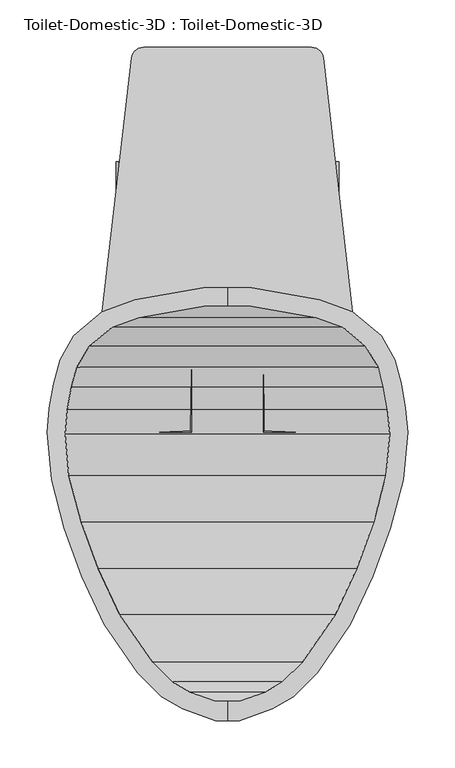
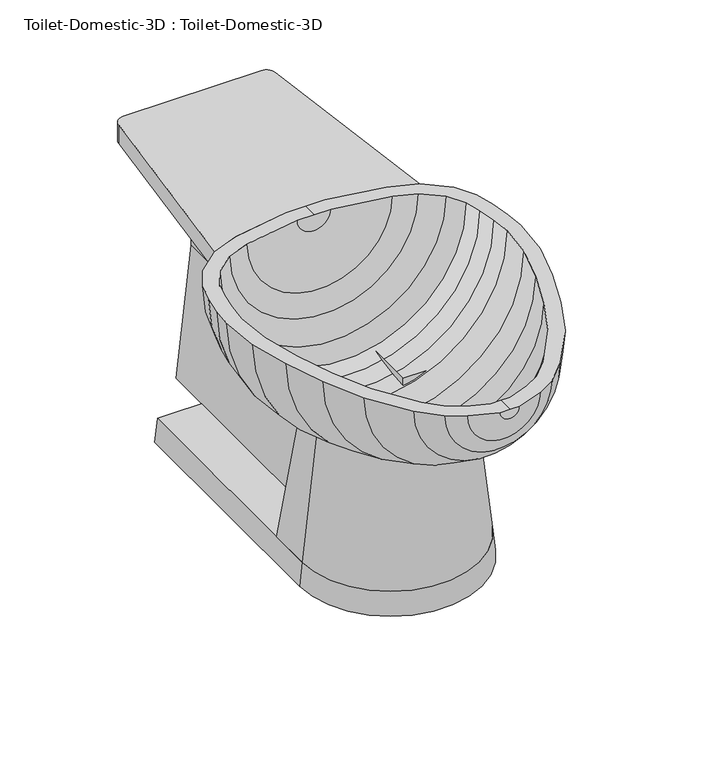
"""IFC4 building model written with IfcOpenShell, lengths in millimetres: flow terminal geometry, Toilet-Domestic-3D : Toilet-Domestic-3D."""

from ifc_helpers import new_model, si_unit, point, frame, frame_2d, origin, place, context, project, spatial, polyline, circle_curve, trimmed, segment, composite_curve, outline, extrude, source, transform, mapped, element, save
from ifc_brep_helpers import plane_surface, revolved_surface, advanced_brep


def toilet_domestic_3d_toilet_domestic_3d_ba6479b0(model_context):
    return source(origin(), model_context, "Body", "SolidModel", [
        advanced_brep(
        [(-25.4, 152.4, 361.95), (-97.4252791, 139.7, 361.95), (-132.3182423, 127.0, 361.95), (-162.5887836, 101.6, 361.95), (-176.9845865, 76.2, 361.95), (-183.790496, 50.8, 361.95), (-188.2862441, 25.3033453, 361.95), (-190.5, 0.0, 361.95), (-186.0724883, -50.6066907, 361.95), (-172.4088722, -101.6, 361.95), (-153.9191843, -152.4, 361.95), (-130.2307553, -203.2, 361.95), (-94.9900085, -254.0, 361.95), (-69.5900085, -279.4, 361.95), (-47.5929632, -292.1, 361.95), (-12.7, -304.8, 361.95), (0.0, -304.8, 361.95), (0.0, -284.592034, 361.95), (-12.5224565, -284.592034, 361.95), (-39.5113323, -274.7688865, 361.95), (-58.4178985, -263.8531754, 361.95), (-79.2146703, -243.0564036, 361.95), (-114.0255101, -192.8761202, 361.95), (-136.654021, -144.3491221, 361.95), (-154.575847, -95.1093097, 361.95), (-167.7238545, -46.0402777, 361.95), (-171.5645445, -2.1409906, 361.95), (-169.3087351, 23.6430284, 361.95), (-165.101298, 47.5045901, 361.95), (-159.5484355, 68.2281551, 361.95), (-146.1085923, 90.5605136, 361.95), (-121.9980886, 110.7916284, 361.95), (-94.1172813, 120.9394123, 361.95), (-22.0920022, 133.6394123, 361.95), (0.0, 133.6394123, 361.95), (0.0, 152.4, 361.95), (25.4, 152.4, 361.95), (22.0920022, 133.6394123, 361.95), (94.1172813, 120.9394123, 361.95), (121.9980886, 110.7916284, 361.95), (146.1085923, 90.5605136, 361.95), (159.5484355, 68.2281551, 361.95), (165.101298, 47.5045901, 361.95), (169.3087351, 23.6430284, 361.95), (171.5645445, -2.1409906, 361.95), (167.7238545, -46.0402777, 361.95), (154.575847, -95.1093097, 361.95), (136.654021, -144.3491221, 361.95), (114.0255101, -192.8761202, 361.95), (79.2146703, -243.0564036, 361.95), (58.4178985, -263.8531754, 361.95), (39.5113323, -274.7688865, 361.95), (12.5224565, -284.592034, 361.95), (12.7, -304.8, 361.95), (47.5929632, -292.1, 361.95), (69.5900085, -279.4, 361.95), (94.9900085, -254.0, 361.95), (130.2307553, -203.2, 361.95), (153.9191843, -152.4, 361.95), (172.4088722, -101.6, 361.95), (186.0724883, -50.6066907, 361.95), (190.5, 0.0, 361.95), (188.2862441, 25.3033453, 361.95), (183.790496, 50.8, 361.95), (176.9845865, 76.2, 361.95), (162.5887836, 101.6, 361.95), (132.3182423, 127.0, 361.95), (97.4252791, 139.7, 361.95)],
        [
            (0, 1),
            (1, 2),
            (2, 3),
            (3, 4),
            (4, 5),
            (5, 6),
            (6, 7),
            (7, 8),
            (8, 9),
            (9, 10),
            (10, 11),
            (11, 12),
            (12, 13),
            (13, 14),
            (14, 15),
            (15, 16),
            (16, 17),
            (17, 18),
            (18, 19),
            (19, 20),
            (20, 21),
            (21, 22),
            (22, 23),
            (23, 24),
            (24, 25),
            (25, 26),
            (26, 27),
            (27, 28),
            (28, 29),
            (29, 30),
            (30, 31),
            (31, 32),
            (32, 33),
            (33, 34),
            (34, 35),
            (35, 0),
            (36, 35),
            (34, 37),
            (37, 38),
            (38, 39),
            (39, 40),
            (40, 41),
            (41, 42),
            (42, 43),
            (43, 44),
            (44, 45),
            (45, 46),
            (46, 47),
            (47, 48),
            (48, 49),
            (49, 50),
            (50, 51),
            (51, 52),
            (52, 17),
            (16, 53),
            (53, 54),
            (54, 55),
            (55, 56),
            (56, 57),
            (57, 58),
            (58, 59),
            (59, 60),
            (60, 61),
            (61, 62),
            (62, 63),
            (63, 64),
            (64, 65),
            (65, 66),
            (66, 67),
            (67, 36),
            (67, 1, circle_curve(frame((0.0, 139.7, 361.95), z_axis=(0.0, 1.0, 0.0), x_axis=(-1.0, 0.0, 0.0)), 97.4252791)),
            (0, 36, circle_curve(frame((0.0, 152.4, 361.95), z_axis=(0.0, -1.0, 0.0), x_axis=(-1.0, 0.0, 0.0)), 25.4)),
            (66, 2, circle_curve(frame((0.0, 127.0, 361.95), z_axis=(0.0, 1.0, 0.0), x_axis=(-1.0, 0.0, 0.0)), 132.3182423)),
            (65, 3, circle_curve(frame((0.0, 101.6, 361.95), z_axis=(0.0, 1.0, 0.0), x_axis=(-1.0, 0.0, 0.0)), 162.5887836)),
            (64, 4, circle_curve(frame((0.0, 76.2, 361.95), z_axis=(0.0, 1.0, 0.0), x_axis=(-1.0, 0.0, 0.0)), 176.9845865)),
            (63, 5, circle_curve(frame((0.0, 50.8, 361.95), z_axis=(0.0, 1.0, 0.0), x_axis=(-1.0, 0.0, 0.0)), 183.790496)),
            (62, 6, circle_curve(frame((0.0, 25.3033453, 361.95), z_axis=(0.0, 1.0, 0.0), x_axis=(-1.0, 0.0, 0.0)), 188.2862441)),
            (61, 7, circle_curve(frame((0.0, 0.0, 361.95), z_axis=(0.0, 1.0, 0.0), x_axis=(-1.0, 0.0, 0.0)), 190.5)),
            (60, 8, circle_curve(frame((0.0, -50.6066907, 361.95), z_axis=(0.0, 1.0, 0.0), x_axis=(-1.0, 0.0, 0.0)), 186.0724883)),
            (59, 9, circle_curve(frame((0.0, -101.6, 361.95), z_axis=(0.0, 1.0, 0.0), x_axis=(-1.0, 0.0, 0.0)), 172.4088722)),
            (58, 10, circle_curve(frame((0.0, -152.4, 361.95), z_axis=(0.0, 1.0, 0.0), x_axis=(-1.0, 0.0, 0.0)), 153.9191843)),
            (57, 11, circle_curve(frame((0.0, -203.2, 361.95), z_axis=(0.0, 1.0, 0.0), x_axis=(-1.0, 0.0, 0.0)), 130.2307553)),
            (56, 12, circle_curve(frame((0.0, -254.0, 361.95), z_axis=(0.0, 1.0, 0.0), x_axis=(-1.0, 0.0, 0.0)), 94.9900085)),
            (55, 13, circle_curve(frame((0.0, -279.4, 361.95), z_axis=(0.0, 1.0, 0.0), x_axis=(-1.0, 0.0, 0.0)), 69.5900085)),
            (54, 14, circle_curve(frame((0.0, -292.1, 361.95), z_axis=(0.0, 1.0, 0.0), x_axis=(-1.0, 0.0, 0.0)), 47.5929632)),
            (53, 15, circle_curve(frame((0.0, -304.8, 361.95), z_axis=(0.0, 1.0, 0.0), x_axis=(-1.0, 0.0, 0.0)), 12.7)),
            (52, 18, circle_curve(frame((0.0, -284.592034, 361.95), z_axis=(0.0, 1.0, 0.0), x_axis=(-1.0, 0.0, 0.0)), 12.5224565)),
            (51, 19, circle_curve(frame((0.0, -274.7688865, 361.95), z_axis=(0.0, 1.0, 0.0), x_axis=(-1.0, 0.0, 0.0)), 39.5113323)),
            (50, 20, circle_curve(frame((0.0, -263.8531754, 361.95), z_axis=(0.0, 1.0, 0.0), x_axis=(-1.0, 0.0, 0.0)), 58.4178985)),
            (49, 21, circle_curve(frame((0.0, -243.0564036, 361.95), z_axis=(0.0, 1.0, 0.0), x_axis=(-1.0, 0.0, 0.0)), 79.2146703)),
            (48, 22, circle_curve(frame((0.0, -192.8761202, 361.95), z_axis=(0.0, 1.0, 0.0), x_axis=(-1.0, 0.0, 0.0)), 114.0255101)),
            (47, 23, circle_curve(frame((0.0, -144.3491221, 361.95), z_axis=(0.0, 1.0, 0.0), x_axis=(-1.0, 0.0, 0.0)), 136.654021)),
            (46, 24, circle_curve(frame((0.0, -95.1093097, 361.95), z_axis=(0.0, 1.0, 0.0), x_axis=(-1.0, 0.0, 0.0)), 154.575847)),
            (45, 25, circle_curve(frame((0.0, -46.0402777, 361.95), z_axis=(0.0, 1.0, 0.0), x_axis=(-1.0, 0.0, 0.0)), 167.7238545)),
            (44, 26, circle_curve(frame((0.0, -2.1409906, 361.95), z_axis=(0.0, 1.0, 0.0), x_axis=(-1.0, 0.0, 0.0)), 171.5645445)),
            (43, 27, circle_curve(frame((0.0, 23.6430284, 361.95), z_axis=(0.0, 1.0, 0.0), x_axis=(-1.0, 0.0, 0.0)), 169.3087351)),
            (42, 28, circle_curve(frame((0.0, 47.5045901, 361.95), z_axis=(0.0, 1.0, 0.0), x_axis=(-1.0, 0.0, 0.0)), 165.101298)),
            (41, 29, circle_curve(frame((0.0, 68.2281551, 361.95), z_axis=(0.0, 1.0, 0.0), x_axis=(-1.0, 0.0, 0.0)), 159.5484355)),
            (40, 30, circle_curve(frame((0.0, 90.5605136, 361.95), z_axis=(0.0, 1.0, 0.0), x_axis=(-1.0, 0.0, 0.0)), 146.1085923)),
            (39, 31, circle_curve(frame((0.0, 110.7916284, 361.95), z_axis=(0.0, 1.0, 0.0), x_axis=(-1.0, 0.0, 0.0)), 121.9980886)),
            (38, 32, circle_curve(frame((0.0, 120.9394123, 361.95), z_axis=(0.0, 1.0, 0.0), x_axis=(-1.0, 0.0, 0.0)), 94.1172813)),
            (37, 33, circle_curve(frame((0.0, 133.6394123, 361.95), z_axis=(0.0, 1.0, 0.0), x_axis=(-1.0, 0.0, 0.0)), 22.0920022)),
        ],
        [
            plane_surface(frame((0.0, 175.1599017, 361.95), z_axis=(0.0, 0.0, 1.0), x_axis=(-1.0, 0.0, 0.0))),
            plane_surface(frame((0.0, 175.1599017, 361.95), z_axis=(0.0, 0.0, 1.0), x_axis=(1.0, 0.0, 0.0))),
            revolved_surface(polyline([(-25.4, 152.4, 361.95), (-97.4252791, 139.7, 361.95)]), (0.0, 175.1599017, 361.95), (0.0, -1.0, 0.0)),
            revolved_surface(polyline([(-97.4252791, 139.7, 361.95), (-132.3182423, 127.0, 361.95)]), (0.0, 175.1599017, 361.95), (0.0, -1.0, 0.0)),
            revolved_surface(polyline([(-132.3182423, 127.0, 361.95), (-162.5887836, 101.6, 361.95)]), (0.0, 175.1599017, 361.95), (0.0, -1.0, 0.0)),
            revolved_surface(polyline([(-162.5887836, 101.6, 361.95), (-176.9845865, 76.2, 361.95)]), (0.0, 175.1599017, 361.95), (0.0, -1.0, 0.0)),
            revolved_surface(polyline([(-176.9845865, 76.2, 361.95), (-183.790496, 50.8, 361.95)]), (0.0, 175.1599017, 361.95), (0.0, -1.0, 0.0)),
            revolved_surface(polyline([(-183.790496, 50.8, 361.95), (-188.2862441, 25.3033453, 361.95)]), (0.0, 175.1599017, 361.95), (0.0, -1.0, 0.0)),
            revolved_surface(polyline([(-188.2862441, 25.3033453, 361.95), (-190.5, 0.0, 361.95)]), (0.0, 175.1599017, 361.95), (0.0, -1.0, 0.0)),
            revolved_surface(polyline([(-190.5, 0.0, 361.95), (-186.0724883, -50.6066907, 361.95)]), (0.0, 175.1599017, 361.95), (0.0, -1.0, 0.0)),
            revolved_surface(polyline([(-186.0724883, -50.6066907, 361.95), (-172.4088722, -101.6, 361.95)]), (0.0, 175.1599017, 361.95), (0.0, -1.0, 0.0)),
            revolved_surface(polyline([(-172.4088722, -101.6, 361.95), (-153.9191843, -152.4, 361.95)]), (0.0, 175.1599017, 361.95), (0.0, -1.0, 0.0)),
            revolved_surface(polyline([(-153.9191843, -152.4, 361.95), (-130.2307553, -203.2, 361.95)]), (0.0, 175.1599017, 361.95), (0.0, -1.0, 0.0)),
            revolved_surface(polyline([(-130.2307553, -203.2, 361.95), (-94.9900085, -254.0, 361.95)]), (0.0, 175.1599017, 361.95), (0.0, -1.0, 0.0)),
            revolved_surface(polyline([(-94.9900085, -254.0, 361.95), (-69.5900085, -279.4, 361.95)]), (0.0, 175.1599017, 361.95), (0.0, -1.0, 0.0)),
            revolved_surface(polyline([(-69.5900085, -279.4, 361.95), (-47.5929632, -292.1, 361.95)]), (0.0, 175.1599017, 361.95), (0.0, -1.0, 0.0)),
            revolved_surface(polyline([(-47.5929632, -292.1, 361.95), (-12.7, -304.8, 361.95)]), (0.0, 175.1599017, 361.95), (0.0, -1.0, 0.0)),
            plane_surface(frame((0.0, -304.8, 361.95), z_axis=(0.0, -1.0, 0.0), x_axis=(-1.0, 0.0, 0.0))),
            plane_surface(frame((0.0, -284.592034, 361.95), z_axis=(0.0, 1.0, 0.0), x_axis=(-1.0, 0.0, 0.0))),
            revolved_surface(polyline([(-12.5224565, -284.592034, 361.95), (-39.5113323, -274.7688865, 361.95)]), (0.0, 175.1599017, 361.95), (0.0, -1.0, 0.0)),
            revolved_surface(polyline([(-39.5113323, -274.7688865, 361.95), (-58.4178985, -263.8531754, 361.95)]), (0.0, 175.1599017, 361.95), (0.0, -1.0, 0.0)),
            revolved_surface(polyline([(-58.4178985, -263.8531754, 361.95), (-79.2146703, -243.0564036, 361.95)]), (0.0, 175.1599017, 361.95), (0.0, -1.0, 0.0)),
            revolved_surface(polyline([(-79.2146703, -243.0564036, 361.95), (-114.0255101, -192.8761202, 361.95)]), (0.0, 175.1599017, 361.95), (0.0, -1.0, 0.0)),
            revolved_surface(polyline([(-114.0255101, -192.8761202, 361.95), (-136.654021, -144.3491221, 361.95)]), (0.0, 175.1599017, 361.95), (0.0, -1.0, 0.0)),
            revolved_surface(polyline([(-136.654021, -144.3491221, 361.95), (-154.575847, -95.1093097, 361.95)]), (0.0, 175.1599017, 361.95), (0.0, -1.0, 0.0)),
            revolved_surface(polyline([(-154.575847, -95.1093097, 361.95), (-167.7238545, -46.0402777, 361.95)]), (0.0, 175.1599017, 361.95), (0.0, -1.0, 0.0)),
            revolved_surface(polyline([(-167.7238545, -46.0402777, 361.95), (-171.5645445, -2.1409906, 361.95)]), (0.0, 175.1599017, 361.95), (0.0, -1.0, 0.0)),
            revolved_surface(polyline([(-171.5645445, -2.1409906, 361.95), (-169.3087351, 23.6430284, 361.95)]), (0.0, 175.1599017, 361.95), (0.0, -1.0, 0.0)),
            revolved_surface(polyline([(-169.3087351, 23.6430284, 361.95), (-165.101298, 47.5045901, 361.95)]), (0.0, 175.1599017, 361.95), (0.0, -1.0, 0.0)),
            revolved_surface(polyline([(-165.101298, 47.5045901, 361.95), (-159.5484355, 68.2281551, 361.95)]), (0.0, 175.1599017, 361.95), (0.0, -1.0, 0.0)),
            revolved_surface(polyline([(-159.5484355, 68.2281551, 361.95), (-146.1085923, 90.5605136, 361.95)]), (0.0, 175.1599017, 361.95), (0.0, -1.0, 0.0)),
            revolved_surface(polyline([(-146.1085923, 90.5605136, 361.95), (-121.9980886, 110.7916284, 361.95)]), (0.0, 175.1599017, 361.95), (0.0, -1.0, 0.0)),
            revolved_surface(polyline([(-121.9980886, 110.7916284, 361.95), (-94.1172813, 120.9394123, 361.95)]), (0.0, 175.1599017, 361.95), (0.0, -1.0, 0.0)),
            revolved_surface(polyline([(-94.1172813, 120.9394123, 361.95), (-22.0920022, 133.6394123, 361.95)]), (0.0, 175.1599017, 361.95), (0.0, -1.0, 0.0)),
            plane_surface(frame((0.0, 133.6394123, 361.95), z_axis=(0.0, -1.0, 0.0), x_axis=(-1.0, 0.0, 0.0))),
            plane_surface(frame((0.0, 152.4, 361.95), z_axis=(0.0, 1.0, 0.0), x_axis=(-1.0, 0.0, 0.0))),
        ],
        [
            (0, [[1, 2, 3, 4, 5, 6, 7, 8, 9, 10, 11, 12, 13, 14, 15, 16, 17, 18, 19, 20, 21, 22, 23, 24, 25, 26, 27, 28, 29, 30, 31, 32, 33, 34, 35, 36]]),
            (1, [[37, -35, 38, 39, 40, 41, 42, 43, 44, 45, 46, 47, 48, 49, 50, 51, 52, 53, 54, -17, 55, 56, 57, 58, 59, 60, 61, 62, 63, 64, 65, 66, 67, 68, 69, 70]]),
            (2, [[71, -1, 72, -70]]),
            (3, [[73, -2, -71, -69]]),
            (4, [[74, -3, -73, -68]]),
            (5, [[75, -4, -74, -67]]),
            (6, [[76, -5, -75, -66]]),
            (7, [[77, -6, -76, -65]]),
            (8, [[78, -7, -77, -64]]),
            (9, [[79, -8, -78, -63]]),
            (10, [[80, -9, -79, -62]]),
            (11, [[81, -10, -80, -61]]),
            (12, [[82, -11, -81, -60]]),
            (13, [[83, -12, -82, -59]]),
            (14, [[84, -13, -83, -58]]),
            (15, [[85, -14, -84, -57]]),
            (16, [[86, -15, -85, -56]]),
            (17, [[-16, -86, -55]]),
            (18, [[87, -18, -54]]),
            (19, [[88, -19, -87, -53]]),
            (20, [[89, -20, -88, -52]]),
            (21, [[90, -21, -89, -51]]),
            (22, [[91, -22, -90, -50]]),
            (23, [[92, -23, -91, -49]]),
            (24, [[93, -24, -92, -48]]),
            (25, [[94, -25, -93, -47]]),
            (26, [[95, -26, -94, -46]]),
            (27, [[96, -27, -95, -45]]),
            (28, [[97, -28, -96, -44]]),
            (29, [[98, -29, -97, -43]]),
            (30, [[99, -30, -98, -42]]),
            (31, [[100, -31, -99, -41]]),
            (32, [[101, -32, -100, -40]]),
            (33, [[102, -33, -101, -39]]),
            (34, [[-34, -102, -38]]),
            (35, [[-72, -36, -37]]),
        ],
    ),
        advanced_brep(
        [(-57.15, 342.9, 31.75), (-38.1, 342.9, 206.375), (-38.1, 342.9, 31.75), (-57.15, 19.05, 31.75), (-38.1, 0.0, 206.375), (-38.1, 0.0, 31.75), (-114.3, 19.05, 31.75), (-95.25, 0.0, 206.375), (-95.25, 0.0, 31.75), (-114.3, -38.1, 31.75), (-95.25, -38.1, 206.375), (-95.25, -38.1, 31.75), (95.25, -38.1, 206.375), (114.3, -38.1, 31.75), (95.25, -38.1, 31.75), (114.3, 19.05, 31.75), (95.25, 0.0, 206.375), (95.25, 0.0, 31.75), (57.15, 19.05, 31.75), (38.1, 0.0, 206.375), (38.1, 0.0, 31.75), (57.15, 342.9, 31.75), (38.1, 342.9, 31.75), (38.1, 342.9, 206.375)],
        [
            (0, 1),
            (1, 2),
            (2, 0),
            (0, 3),
            (3, 4),
            (4, 1),
            (4, 5),
            (5, 2),
            (5, 3),
            (3, 6),
            (6, 7),
            (7, 4),
            (7, 8),
            (8, 5),
            (8, 6),
            (6, 9),
            (9, 10),
            (10, 7),
            (10, 11),
            (11, 8),
            (11, 9),
            (12, 10, circle_curve(frame((0.0, -38.1, 206.375), z_axis=(0.0, 0.0, -1.0), x_axis=(-1.0, 0.0, 0.0)), 95.25)),
            (9, 13, circle_curve(frame((0.0, -38.1, 31.75), z_axis=(0.0, 0.0, 1.0), x_axis=(-1.0, 0.0, 0.0)), 114.3)),
            (13, 12),
            (14, 11, circle_curve(frame((0.0, -38.1, 31.75), z_axis=(0.0, 0.0, -1.0), x_axis=(-1.0, 0.0, 0.0)), 95.25)),
            (12, 14),
            (14, 13),
            (13, 15),
            (15, 16),
            (16, 12),
            (16, 17),
            (17, 14),
            (17, 15),
            (15, 18),
            (18, 19),
            (19, 16),
            (19, 20),
            (20, 17),
            (20, 18),
            (21, 22),
            (22, 23),
            (23, 21),
            (18, 21),
            (23, 19),
            (22, 20),
        ],
        [
            plane_surface(frame((-244.475, 342.9, 0.0), z_axis=(0.0, 1.0, 0.0), x_axis=(0.0, 0.0, -1.0))),
            plane_surface(frame((-57.15, 342.9, 31.75), z_axis=(-0.9941021766079944, 0.0, 0.10844751017542063), x_axis=(0.0, -1.0, 0.0))),
            plane_surface(frame((-38.1, 342.9, 206.375), z_axis=(1.0, 0.0, 0.0), x_axis=(0.0, -1.0, 0.0))),
            plane_surface(frame((-38.1, 342.9, 31.75), z_axis=(0.0, 0.0, -1.0), x_axis=(0.0, -1.0, 0.0))),
            plane_surface(frame((-57.15, 19.05, 31.75), z_axis=(0.0, 0.9941021766079944, 0.10844751017542063), x_axis=(-1.0, 0.0, 0.0))),
            plane_surface(frame((-38.1, 0.0, 206.375), z_axis=(0.0, -1.0, 0.0), x_axis=(-1.0, 0.0, 0.0))),
            plane_surface(frame((-38.1, 0.0, 31.75), z_axis=(0.0, 0.0, -1.0), x_axis=(-1.0, 0.0, 0.0))),
            plane_surface(frame((-114.3, 19.05, 31.75), z_axis=(-0.9941021766079944, 0.0, 0.10844751017542063), x_axis=(0.0, -1.0, 0.0))),
            plane_surface(frame((-95.25, 0.0, 206.375), z_axis=(1.0, 0.0, 0.0), x_axis=(0.0, -1.0, 0.0))),
            plane_surface(frame((-95.25, 0.0, 31.75), z_axis=(0.0, 0.0, -1.0), x_axis=(0.0, -1.0, 0.0))),
            revolved_surface(polyline([(-114.3, -38.1, 31.75), (-95.25, -38.1, 206.375)]), (0.0, -38.1, 0.0), (0.0, 0.0, 1.0)),
            revolved_surface(polyline([(-95.25, -38.1, 206.375), (-95.25, -38.1, 31.75)]), (0.0, -38.1, 0.0), (0.0, 0.0, 1.0)),
            plane_surface(frame((0.0, -38.1, 31.75), z_axis=(0.0, 0.0, -1.0), x_axis=(-1.0, 0.0, 0.0))),
            plane_surface(frame((114.3, -38.1, 31.75), z_axis=(0.9941021766079944, 0.0, 0.10844751017542063), x_axis=(0.0, 1.0, 0.0))),
            plane_surface(frame((95.25, -38.1, 206.375), z_axis=(-1.0, 0.0, 0.0), x_axis=(0.0, 1.0, 0.0))),
            plane_surface(frame((95.25, -38.1, 31.75), z_axis=(0.0, 0.0, -1.0), x_axis=(0.0, 1.0, 0.0))),
            plane_surface(frame((114.3, 19.05, 31.75), z_axis=(0.0, 0.9941021766079944, 0.10844751017542063), x_axis=(-1.0, 0.0, 0.0))),
            plane_surface(frame((95.25, 0.0, 206.375), z_axis=(0.0, -1.0, 0.0), x_axis=(-1.0, 0.0, 0.0))),
            plane_surface(frame((95.25, 0.0, 31.75), z_axis=(0.0, 0.0, -1.0), x_axis=(-1.0, 0.0, 0.0))),
            plane_surface(frame((-168.275, 342.9, 0.0), z_axis=(0.0, 1.0, 0.0), x_axis=(0.0, 0.0, 1.0))),
            plane_surface(frame((57.15, 19.05, 31.75), z_axis=(0.9941021766079944, 0.0, 0.10844751017542063), x_axis=(0.0, 1.0, 0.0))),
            plane_surface(frame((38.1, 0.0, 206.375), z_axis=(-1.0, 0.0, 0.0), x_axis=(0.0, 1.0, 0.0))),
            plane_surface(frame((38.1, 0.0, 31.75), z_axis=(0.0, 0.0, -1.0), x_axis=(0.0, 1.0, 0.0))),
        ],
        [
            (0, [[1, 2, 3]]),
            (1, [[-1, 4, 5, 6]]),
            (2, [[-2, -6, 7, 8]]),
            (3, [[-3, -8, 9, -4]]),
            (4, [[-5, 10, 11, 12]]),
            (5, [[-7, -12, 13, 14]]),
            (6, [[-9, -14, 15, -10]]),
            (7, [[-11, 16, 17, 18]]),
            (8, [[-13, -18, 19, 20]]),
            (9, [[-15, -20, 21, -16]]),
            (10, [[22, -17, 23, 24]]),
            (11, [[25, -19, -22, 26]]),
            (12, [[-23, -21, -25, 27]]),
            (13, [[-24, 28, 29, 30]]),
            (14, [[-26, -30, 31, 32]]),
            (15, [[-27, -32, 33, -28]]),
            (16, [[-29, 34, 35, 36]]),
            (17, [[-31, -36, 37, 38]]),
            (18, [[-33, -38, 39, -34]]),
            (19, [[40, 41, 42]]),
            (20, [[-35, 43, -42, 44]]),
            (21, [[-37, -44, -41, 45]]),
            (22, [[-39, -45, -40, -43]]),
        ],
    ),
        advanced_brep(
        [(-117.7636364, 285.75, 0.0), (-114.3, 285.75, 31.75), (-38.1, 285.75, 31.75), (-38.1, 285.75, 0.0), (-117.7636364, -38.0999951, 0.0), (-114.3, -38.0999951, 31.75), (-38.1, -38.0999951, 31.75), (-38.1, -38.0999951, 0.0), (114.2999707, -38.0999951, 31.75), (117.7636071, -38.0999951, 0.0), (38.0999707, -38.0999951, 31.75), (38.0999707, -38.0999951, 0.0), (117.7636071, 285.6681634, 0.0), (38.0999707, 285.6681634, 0.0), (38.0999707, 285.6681634, 31.75), (114.2999707, 285.6681634, 31.75)],
        [
            (0, 1),
            (1, 2),
            (2, 3),
            (3, 0),
            (0, 4),
            (4, 5),
            (5, 1),
            (5, 6),
            (6, 2),
            (6, 7),
            (7, 3),
            (7, 4),
            (8, 5, circle_curve(frame((-1.46e-05, -38.0999951, 31.75), z_axis=(0.0, 0.0, -1.0), x_axis=(-1.0, 0.0, 0.0)), 114.2999854)),
            (4, 9, circle_curve(frame((-1.46e-05, -38.0999951, 0.0), z_axis=(0.0, 0.0, 1.0), x_axis=(-1.0, 0.0, 0.0)), 117.7636217)),
            (9, 8),
            (10, 6, circle_curve(frame((-1.46e-05, -38.0999951, 31.75), z_axis=(0.0, 0.0, -1.0), x_axis=(-1.0, 0.0, 0.0)), 38.0999854)),
            (8, 10),
            (11, 7, circle_curve(frame((-1.46e-05, -38.0999951, 0.0), z_axis=(0.0, 0.0, -1.0), x_axis=(-1.0, 0.0, 0.0)), 38.0999854)),
            (10, 11),
            (11, 9),
            (12, 13),
            (13, 14),
            (14, 15),
            (15, 12),
            (9, 12),
            (15, 8),
            (14, 10),
            (13, 11),
        ],
        [
            plane_surface(frame((-196.85, 285.75, 0.0), z_axis=(0.0, 1.0, 0.0), x_axis=(0.0, 0.0, -1.0))),
            plane_surface(frame((-117.7636364, 285.75, 0.0), z_axis=(-0.9941021766079929, 0.0, 0.10844751017543448), x_axis=(0.0, -1.0, 0.0))),
            plane_surface(frame((-114.3, 285.75, 31.75), z_axis=(0.0, 0.0, 1.0), x_axis=(0.0, -1.0, 0.0))),
            plane_surface(frame((-38.1, 285.75, 31.75), z_axis=(1.0, 0.0, 0.0), x_axis=(0.0, -1.0, 0.0))),
            plane_surface(frame((-38.1, 285.75, 0.0), z_axis=(0.0, 0.0, -1.0), x_axis=(0.0, -1.0, 0.0))),
            revolved_surface(polyline([(-117.7636364, -38.0999951, 0.0), (-114.3, -38.0999951, 31.75)]), (-1.46e-05, -38.0999951, 0.0), (0.0, 0.0, 1.0)),
            plane_surface(frame((-1.46e-05, -38.0999951, 31.75), z_axis=(0.0, 0.0, 1.0), x_axis=(-1.0, 0.0, 0.0))),
            revolved_surface(polyline([(-38.1, -38.0999951, 31.75), (-38.1, -38.0999951, 0.0)]), (-1.46e-05, -38.0999951, 0.0), (0.0, 0.0, 1.0)),
            plane_surface(frame((-1.46e-05, -38.0999951, 0.0), z_axis=(0.0, 0.0, -1.0), x_axis=(-1.0, 0.0, 0.0))),
            plane_surface(frame((31.7499707, 285.6681634, 0.0), z_axis=(0.0, 1.0, 0.0), x_axis=(0.0, 0.0, 1.0))),
            plane_surface(frame((117.7636071, -38.0999951, 0.0), z_axis=(0.9941021766079929, 0.0, 0.10844751017543448), x_axis=(0.0, 1.0, 0.0))),
            plane_surface(frame((114.2999707, -38.0999951, 31.75), z_axis=(0.0, 0.0, 1.0), x_axis=(0.0, 1.0, 0.0))),
            plane_surface(frame((38.0999707, -38.0999951, 31.75), z_axis=(-1.0, 0.0, 0.0), x_axis=(0.0, 1.0, 0.0))),
            plane_surface(frame((38.0999707, -38.0999951, 0.0), z_axis=(0.0, 0.0, -1.0), x_axis=(0.0, 1.0, 0.0))),
        ],
        [
            (0, [[1, 2, 3, 4]]),
            (1, [[-1, 5, 6, 7]]),
            (2, [[-2, -7, 8, 9]]),
            (3, [[-3, -9, 10, 11]]),
            (4, [[-4, -11, 12, -5]]),
            (5, [[13, -6, 14, 15]]),
            (6, [[16, -8, -13, 17]]),
            (7, [[18, -10, -16, 19]]),
            (8, [[-14, -12, -18, 20]]),
            (9, [[21, 22, 23, 24]]),
            (10, [[-15, 25, -24, 26]]),
            (11, [[-17, -26, -23, 27]]),
            (12, [[-19, -27, -22, 28]]),
            (13, [[-20, -28, -21, -25]]),
        ],
    ),
        extrude(outline(polyline([(139.7, 264.5247209), (152.4, 336.55), (342.9, 336.55), (342.9, 206.375), (107.4852632, 206.375), (127.0, 229.6317577), (139.7, 264.5247209)])), frame((-38.1, 0.0, 0.0), z_axis=(1.0, 0.0, 0.0), x_axis=(0.0, 1.0, 0.0)), (0.0, 0.0, 1.0), 76.2),
        extrude(outline(composite_curve([segment(polyline([(-25.4, 152.4), (-97.4252791, 139.7), (-132.3182423, 127.0), (-101.4824733, 395.1508638)]), True, "CONTINUOUS"), segment(trimmed(circle_curve(frame_2d((-88.8656197, 393.7)), 12.7), [point((-101.4824733, 395.1508638))], [point((-88.8656197, 406.4))], False, "CARTESIAN"), True, "CONTINUOUS"), segment(polyline([(-88.8656197, 406.4), (88.8656197, 406.4)]), True, "CONTINUOUS"), segment(trimmed(circle_curve(frame_2d((88.8656197, 393.7)), 12.7), [point((88.8656197, 406.4))], [point((101.4824733, 395.1508638))], False, "CARTESIAN"), True, "CONTINUOUS"), segment(polyline([(101.4824733, 395.1508638), (132.3182423, 127.0), (97.4252791, 139.7), (25.4, 152.4), (0.0, 152.4), (-25.4, 152.4)]), True, "CONTINUOUS")], self_intersect=False)), frame((0.0, 0.0, 336.55), z_axis=(0.0, 0.0, 1.0), x_axis=(1.0, 0.0, 0.0)), (0.0, 0.0, 1.0), 25.4),
    ])


if __name__ == "__main__":
    model = new_model("IFC4")
    model_context = context("Model", 3, world=origin())
    ifc_project = project(units=[si_unit("LENGTHUNIT", "METRE", prefix="MILLI")], contexts=[model_context])
    site = spatial("IfcSite", under=ifc_project)
    building = spatial("IfcBuilding", under=site)
    placement = place(None, origin())
    toilet_domestic_3d_toilet_domestic_3d_shape = toilet_domestic_3d_toilet_domestic_3d_ba6479b0(model_context)
    element("IfcFlowTerminal", 1, ObjectType="Toilet-Domestic-3D : Toilet-Domestic-3D", at=placement, inside=building, context=model_context, shape_type="MappedRepresentation", body=[
        mapped(toilet_domestic_3d_toilet_domestic_3d_shape, transform((0.0, 0.0, 0.0), x_axis=(1.0, 0.0, 0.0), y_axis=(0.0, 1.0, 0.0), z_axis=(0.0, 0.0, 1.0))),
    ])
    save(model, "model.ifc")

# Revit data of these elements
# Type "Toilet-Domestic-3D : Toilet-Domestic-3D"
#   Assembly Code = "D2010110"
#   Toilet - Bowl/Basin Material = Porcelain, Linen
#   Toilet - Seat Material = Laminate, Linen, Matte
#   Default Elevation = 0
# Element 1 (IfcFlowTerminal, "Toilet-Domestic-3D : Toilet-Domestic-3D")
#   Materials on its faces: "Porcelain, Linen", "Laminate, Linen, Matte"
# Materials
#   "Porcelain, Linen": class "Ceramic", colour RGB 249 239 230, transparency 0, Description = "Porcelain, linen", Cost = 0
#   "Laminate, Linen, Matte": class "Plastic", colour RGB 249 239 230, transparency 0, Description = "Plastic Laminate - Linen, Matte", Cost = 0
